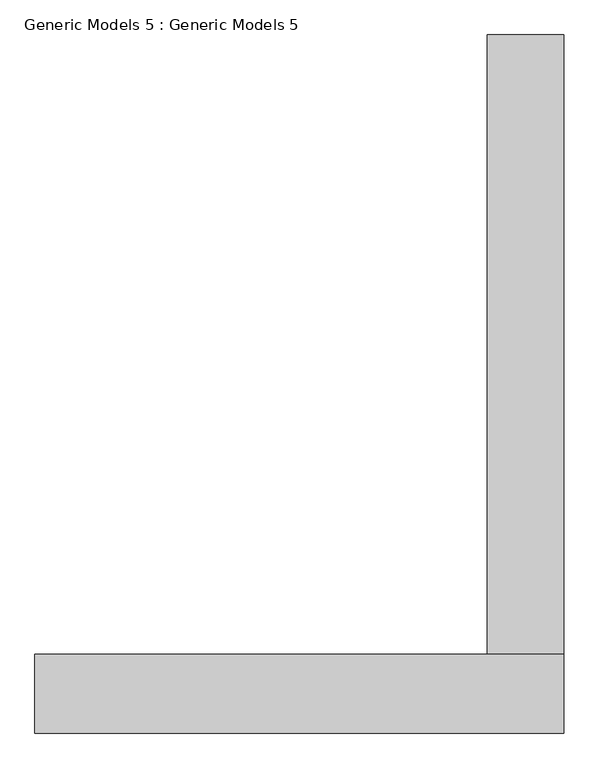
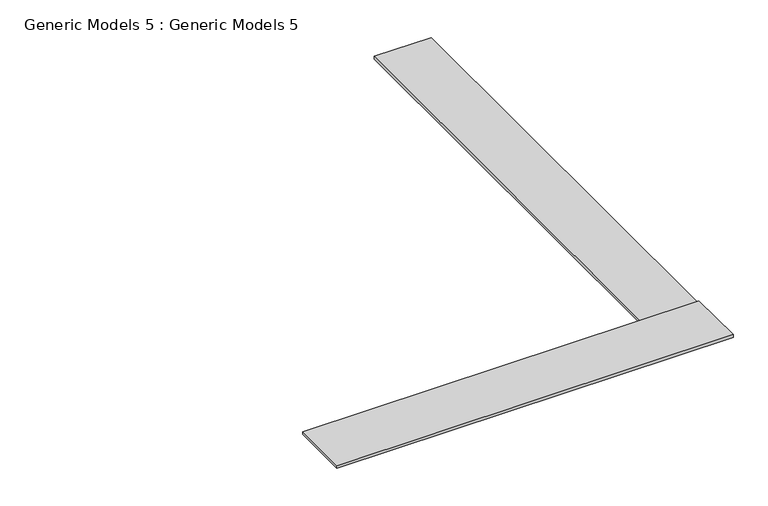
"""IFC4 building model written with IfcOpenShell, lengths in millimetres: proxy geometry, Generic Models 5 : Generic Models 5."""

from ifc_helpers import new_model, si_unit, frame, origin, origin_with_axes, place, context, project, spatial, polyline, outline, extrude, source, transform, mapped, element, save


def generic_models_5_generic_models_5_1652e53f(model_context):
    return source(origin(), model_context, "Body", "SweptSolid", [
        extrude(outline(polyline([(7981.5217545, -10542.3830082), (7981.5217545, 14832.8060031), (11102.3322514, 14832.8060031), (11102.3322514, -10542.3830082), (7981.5217545, -10542.3830082)])), frame((0.0, 0.0, -152.4), z_axis=(0.0, 0.0, 1.0), x_axis=(1.0, 0.0, 0.0)), (0.0, 0.0, 1.0), 152.4),
        extrude(outline(polyline([(11102.3322514, -13777.8442098), (-10564.7066207, -13777.8442098), (-10564.7066207, -10542.3830082), (11102.3322514, -10542.3830082), (11102.3322514, -13777.8442098)])), origin_with_axes(), (0.0, 0.0, 1.0), 152.4),
    ])


if __name__ == "__main__":
    model = new_model("IFC4")
    model_context = context("Model", 3, world=origin())
    ifc_project = project(units=[si_unit("LENGTHUNIT", "METRE", prefix="MILLI")], contexts=[model_context])
    site = spatial("IfcSite", under=ifc_project)
    building = spatial("IfcBuilding", under=site)
    placement = place(None, origin())
    generic_models_5_generic_models_5_shape = generic_models_5_generic_models_5_1652e53f(model_context)
    element("IfcBuildingElementProxy", 1, Name="Generic Models 5 : Generic Models 5", ObjectType="Generic Models 5 : Generic Models 5", at=placement, inside=building, context=model_context, shape_type="MappedRepresentation", body=[
        mapped(generic_models_5_generic_models_5_shape, transform((0.0, 0.0, 0.0), x_axis=(1.0, 0.0, 0.0), y_axis=(0.0, 1.0, 0.0), z_axis=(0.0, 0.0, 1.0))),
    ])
    save(model, "model.ifc")
